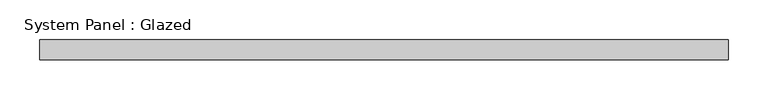
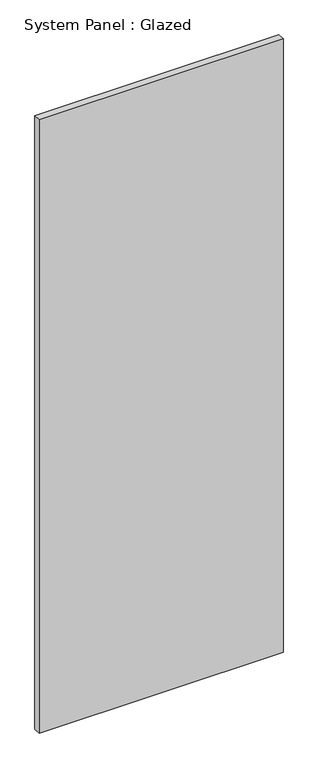
"""IFC4 building model written with IfcOpenShell, lengths in millimetres: plate geometry, System Panel : Glazed."""

from ifc_helpers import new_model, si_unit, origin, origin_with_axes, place, context, project, spatial, polyline, outline, extrude, source, transform, mapped, element, save


def system_panel_glazed_9c94e0d4(model_context):
    return source(origin(), model_context, "Body", "SweptSolid", [
        extrude(outline(polyline([(434.975, 19.05), (-434.975, 19.05), (-434.975, 44.45), (434.975, 44.45), (434.975, 19.05)])), origin_with_axes(), (0.0, 0.0, 1.0), 2311.4),
    ])


if __name__ == "__main__":
    model = new_model("IFC4")
    model_context = context("Model", 3, world=origin())
    ifc_project = project(units=[si_unit("LENGTHUNIT", "METRE", prefix="MILLI")], contexts=[model_context])
    site = spatial("IfcSite", under=ifc_project)
    building = spatial("IfcBuilding", under=site)
    placement = place(None, origin())
    system_panel_glazed_shape = system_panel_glazed_9c94e0d4(model_context)
    element("IfcPlate", 1, ObjectType="System Panel : Glazed", at=placement, inside=building, context=model_context, shape_type="MappedRepresentation", body=[
        mapped(system_panel_glazed_shape, transform((0.0, 0.0, 0.0), x_axis=(1.0, 0.0, 0.0), y_axis=(0.0, 1.0, 0.0), z_axis=(0.0, 0.0, 1.0))),
    ])
    save(model, "model.ifc")

# Revit data of these elements
# Type "System Panel : Glazed"
#   Construction Type Id = "GSP4R"
#   Analytic Construction = "1/8 in Pilkington single glazing"
#   Visual Light Transmittance = 0.9
#   Solar Heat Gain Coefficient = 0.86
#   Heat Transfer Coefficient (U) = 1.18115 BTU/(h·ft²·°F)
# Element 1 (IfcPlate, "System Panel : Glazed")
#   Materials on its faces: "Glass"
# Materials
#   "Glass": class "Glass", colour RGB 0 128 192, transparency 0.75, Description = "Soda Lime Glass", Cost = 0
